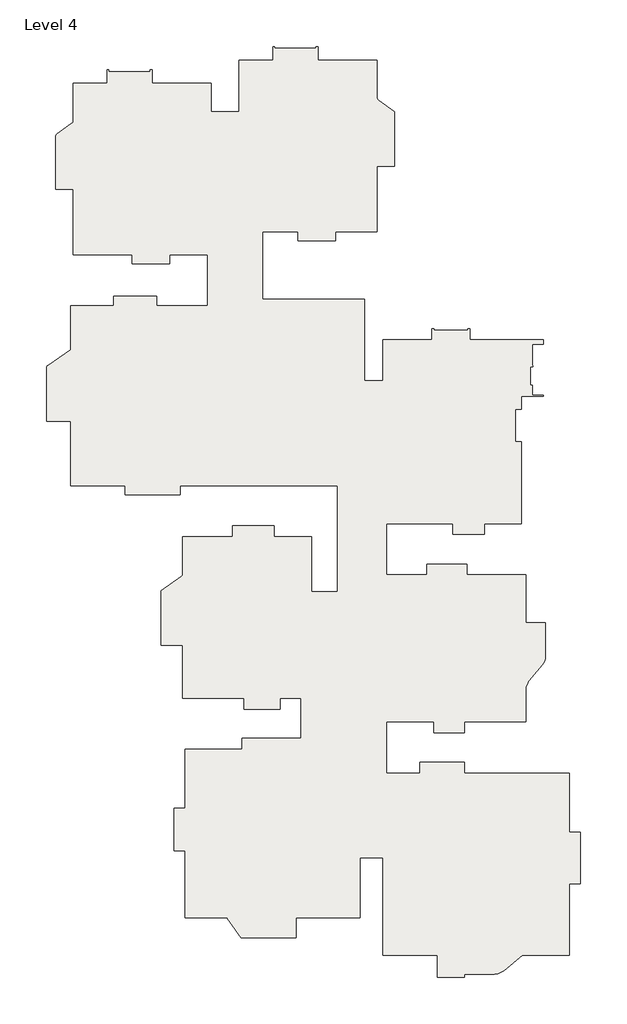
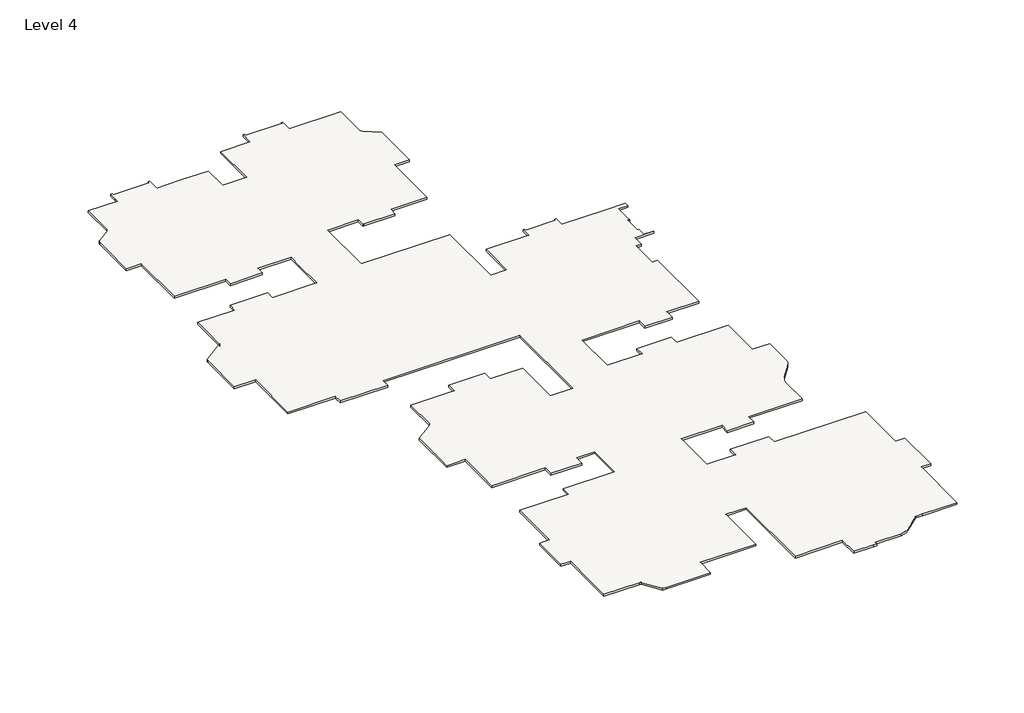
# One storey: 1 slab.
"""IFC4 building model written with IfcOpenShell, lengths in millimetres."""

from ifc_helpers import new_model, si_unit, point, frame, frame_2d, origin, place, context, project, spatial, polyline, circle_curve, trimmed, segment, composite_curve, outline, extrude, element, save

model = new_model("IFC4")

# Units and contexts
model_context = context("Model", 3, world=origin())
ifc_project = project(units=[si_unit("LENGTHUNIT", "METRE", prefix="MILLI")], contexts=[model_context])

# Site, building, storey
site = spatial("IfcSite", under=ifc_project)
building = spatial("IfcBuilding", under=site)
storey = spatial("IfcBuildingStorey", under=building, Name="Level 4", Elevation=6248.4)

# Slab
placement = place(None, origin())
element("IfcSlab", 1, ObjectType="6\" floor", at=placement, inside=storey, context=model_context, shape_type="SweptSolid", body=[
    extrude(outline(composite_curve([segment(polyline([(-9674.5009469, 28521.6416831), (-9674.5009469, 28648.2095876), (-9560.2009469, 28648.2095876), (-9560.2009469, 27756.1461172), (-8800.3399989, 27756.1461172), (-7581.1399989, 27756.1461172), (-5674.0009469, 27756.1461172), (-5674.0009469, 25878.7255084), (-3845.2009469, 25878.7255084), (-3845.2009469, 29269.6255084), (-1617.8862554, 29269.6255084), (-1617.8862554, 30161.6889788), (-1503.5862554, 30161.6889788), (-1503.5862554, 30035.1210743), (1222.0990531, 30035.1210743), (1222.0990531, 30161.6889788), (1336.3990531, 30161.6889788), (1336.3990531, 29269.6255084), (5222.5990531, 29269.6255084), (5222.5990531, 26796.9645799)]), True, "CONTINUOUS"), segment(trimmed(circle_curve(frame_2d((5425.7990531, 26796.9645799)), 203.2), [point((5222.5990531, 26796.9645799))], [point((5309.2715047, 26630.4966536))], True, "CARTESIAN"), True, "CONTINUOUS"), segment(polyline([(5309.2715047, 26630.4966536), (6365.5990531, 25891.0673698), (6365.5990531, 22297.3255084), (5222.5990531, 22297.3255084), (5222.5990531, 18017.4255084), (2479.3990531, 18017.4255084), (2479.3990531, 17431.8689406), (155.2990531, 17431.8689406), (40.9990531, 17431.8689406), (40.9990531, 18017.4255084), (-2288.081873, 18017.4255084), (-2288.081873, 13571.4182723), (4397.0990531, 13571.4182723), (4397.0990531, 8236.2461172), (5616.2990531, 8236.2461172), (5616.2990531, 10928.6450962), (8826.8620119, 10928.6450962), (8826.8620119, 11630.4346228), (8941.1620119, 11630.4346228), (8941.1620119, 11538.2450962), (11198.7752516, 11538.2450962), (11198.7752516, 11630.4346228), (11313.0752516, 11630.4346228), (11313.0752516, 10928.6450962), (14684.0990531, 10928.6450962), (16124.6398221, 10928.6450962), (16124.6398221, 10623.8450962), (15407.9990531, 10623.8450962), (15407.9990531, 9198.1565309), (15440.8254038, 9198.1565309), (15440.8254038, 9147.3565309), (15293.6990531, 9147.3565309), (15293.6990531, 7928.1565309), (15407.9990531, 7928.1565309), (15407.9990531, 7268.4875764), (16124.6398221, 7268.4875764), (16124.6398221, 7211.3375764), (14684.0990531, 7211.3375764), (14684.0990531, 6369.3461172), (14303.0990531, 6369.3461172), (14303.0990531, 5989.8129861), (14303.0990531, 4235.7461172), (14684.0990531, 4235.7461172), (14684.0990531, -1150.3497229), (12281.5704937, -1150.3497229), (12281.5704937, -1861.5497229), (10207.1414203, -1861.5497229), (10207.1414203, -1150.3497229), (5844.8990531, -1150.3497229), (5844.8990531, -4503.1497229), (8478.6664082, -4503.1497229), (8478.6664082, -3803.3538828), (11102.6990531, -3803.3538828), (11102.6990531, -4503.1497229), (14988.8990531, -4503.1497229), (14988.8990531, -7665.4497229), (16284.2990531, -7665.4497229), (16284.2990531, -9831.602777)]), True, "CONTINUOUS"), segment(trimmed(circle_curve(frame_2d((15369.8990531, -9831.602777)), 914.4), [point((16284.2990531, -9831.602777))], [point((16075.314258, -10413.4246987))], False, "CARTESIAN"), True, "CONTINUOUS"), segment(polyline([(16075.314258, -10413.4246987), (15197.8838481, -11477.2429037)]), True, "CONTINUOUS"), segment(trimmed(circle_curve(frame_2d((15903.2990531, -12059.0648255)), 914.4), [point((15197.8838481, -11477.2429037))], [point((14988.8990531, -12059.0648255))], True, "CARTESIAN"), True, "CONTINUOUS"), segment(polyline([(14988.8990531, -12059.0648255), (14988.8990531, -14167.8497229), (10937.0055378, -14167.8497229), (10937.0055378, -14879.0497229), (8943.6990531, -14879.0497229), (8943.6990531, -14167.8497229), (5844.8990531, -14167.8497229), (5844.8990531, -17520.6497229), (8028.4305674, -17520.6497229), (8028.4305674, -16809.4497229), (10950.2990531, -16809.4497229), (10950.2990531, -17520.6497229), (17846.3990531, -17520.6497229), (17846.3990531, -21406.8497229), (18557.5990531, -21406.8497229), (18557.5990531, -24797.7497229), (17846.3990531, -24797.7497229), (17846.3990531, -29484.0497229), (15255.5990531, -29484.0497229), (14750.9761043, -29484.0497229), (13536.5708908, -30485.6833283)]), True, "CONTINUOUS"), segment(trimmed(circle_curve(frame_2d((12809.2934887, -29603.9143222)), 1143.0), [point((13536.5708908, -30485.6833283))], [point((12921.9420983, -30741.3497229))], False, "CARTESIAN"), True, "CONTINUOUS"), segment(polyline([(12921.9420983, -30741.3497229), (10950.2990531, -30741.3497229), (10950.2990531, -30936.1779934), (10721.6990531, -30936.1779934), (9197.6990531, -30936.1779934), (9197.6990531, -29484.0497229), (5616.2990531, -29484.0497229), (5616.2990531, -23083.8583639), (4079.5990531, -23083.8583639), (4079.5990531, -27006.2538828), (-111.4009469, -27006.2538828), (-111.4009469, -28339.7538828), (-3426.1009469, -28339.7538828), (-3705.1428083, -28339.7538828), (-4593.0897712, -27071.2582215)]), True, "CONTINUOUS"), segment(trimmed(circle_curve(frame_2d((-4717.9407159, -27158.6538828)), 152.4), [point((-4593.0897712, -27071.2582215))], [point((-4717.9407159, -27006.2538828))], True, "CARTESIAN"), True, "CONTINUOUS"), segment(polyline([(-4717.9407159, -27006.2538828), (-7388.5009469, -27006.2538828), (-7388.5009469, -22629.8863256), (-8112.4009469, -22629.8863256), (-8112.4009469, -19843.4538828), (-7388.5009469, -19843.4538828), (-7388.5009469, -15957.2538828), (-3654.7009469, -15957.2538828), (-3654.7009469, -15233.3538828), (231.4990531, -15233.3538828), (231.4990531, -12604.4538828), (-1152.8009469, -12604.4538828), (-1152.8009469, -13328.3538828), (-3515.0009469, -13328.3538828), (-3515.0009469, -12604.4538828), (-7553.6009469, -12604.4538828), (-7553.6009469, -9137.3538828), (-8963.3009469, -9137.3538828), (-8963.3009469, -5543.6120214), (-7618.6052856, -4602.3250585)]), True, "CONTINUOUS"), segment(trimmed(circle_curve(frame_2d((-7706.0009469, -4477.4741138)), 152.4), [point((-7618.6052856, -4602.3250585))], [point((-7553.6009469, -4477.4741138))], True, "CARTESIAN"), True, "CONTINUOUS"), segment(polyline([(-7553.6009469, -4477.4741138), (-7553.6009469, -2012.6538828), (-4277.0009469, -2012.6538828), (-4277.0009469, -1288.7538828), (-1533.8009469, -1288.7538828), (-1533.8009469, -2012.6538828), (904.5990531, -2012.6538828), (904.5990531, -5632.1538828), (2631.7990531, -5632.1538828), (2631.7990531, 1340.1461172), (-7726.7333092, 1340.1461172), (-7726.7333092, 730.5461172), (-11312.8009469, 730.5461172), (-11312.8009469, 1340.1461172), (-14894.2009469, 1340.1461172), (-14894.2009469, 5569.2461172), (-16494.4009469, 5569.2461172), (-16494.4009469, 9057.1907685)]), True, "CONTINUOUS"), segment(trimmed(circle_curve(frame_2d((-16291.2009469, 9057.1907685)), 203.2), [point((-16494.4009469, 9057.1907685))], [point((-16407.7284953, 9223.6586947))], False, "CARTESIAN"), True, "CONTINUOUS"), segment(polyline([(-16407.7284953, 9223.6586947), (-14915.8690598, 10267.9602996)]), True, "CONTINUOUS"), segment(trimmed(circle_curve(frame_2d((-14945.0009469, 10309.5772811)), 50.8), [point((-14915.8690598, 10267.9602996))], [point((-14894.2009469, 10309.5772811))], True, "CARTESIAN"), True, "CONTINUOUS"), segment(polyline([(-14894.2009469, 10309.5772811), (-14894.2009469, 13151.1461172), (-12085.9698258, 13151.1461172), (-12085.9698258, 13760.7461172), (-9255.4009469, 13760.7461172), (-9255.4009469, 13151.1461172), (-5902.6009469, 13151.1461172), (-5902.6009469, 15437.1461172), (-5902.6009469, 16503.9461172), (-8417.2009469, 16503.9461172), (-8417.2009469, 15918.3895495), (-10855.6009469, 15918.3895495), (-10855.6009469, 16503.9461172), (-14741.8009469, 16503.9461172), (-14741.8009469, 20783.8461172), (-15884.8009469, 20783.8461172), (-15884.8009469, 24271.7907685)]), True, "CONTINUOUS"), segment(trimmed(circle_curve(frame_2d((-15681.6009469, 24271.7907685)), 203.2), [point((-15884.8009469, 24271.7907685))], [point((-15798.1284953, 24438.2586947))], False, "CARTESIAN"), True, "CONTINUOUS"), segment(polyline([(-15798.1284953, 24438.2586947), (-14828.4733986, 25117.0172625)]), True, "CONTINUOUS"), segment(trimmed(circle_curve(frame_2d((-14945.0009469, 25283.4851887)), 203.2), [point((-14828.4733986, 25117.0172625))], [point((-14741.8009469, 25283.4851887))], True, "CARTESIAN"), True, "CONTINUOUS"), segment(polyline([(-14741.8009469, 25283.4851887), (-14741.8009469, 27756.1461172), (-12514.4862554, 27756.1461172), (-12514.4862554, 28060.9461172), (-12514.4862554, 28648.2095876), (-12400.1862554, 28648.2095876), (-12400.1862554, 28521.6416831), (-9674.5009469, 28521.6416831)]), True, "CONTINUOUS")], self_intersect=False)), frame((0.0, 0.0, 6248.4), z_axis=(0.0, 0.0, 1.0), x_axis=(1.0, 0.0, 0.0)), (0.0, 0.0, 1.0), 152.4),
])

save(model, "model.ifc")

# Revit data of these elements
# Type "6\" floor"
#   Assembly Code = "B1010"
#   Function = 0
#   Layers, outside or top first: 0' - 6" no material (function 1)
# Element 1 (IfcSlab, "6\" floor")
#   Height Offset From Level = 0' - 6"
#   Phase Created = New Construction
#   Materials on its faces: "Default Floor"
# Materials
#   "Default Floor": colour RGB 128 128 128, transparency 0, Cost = 0
